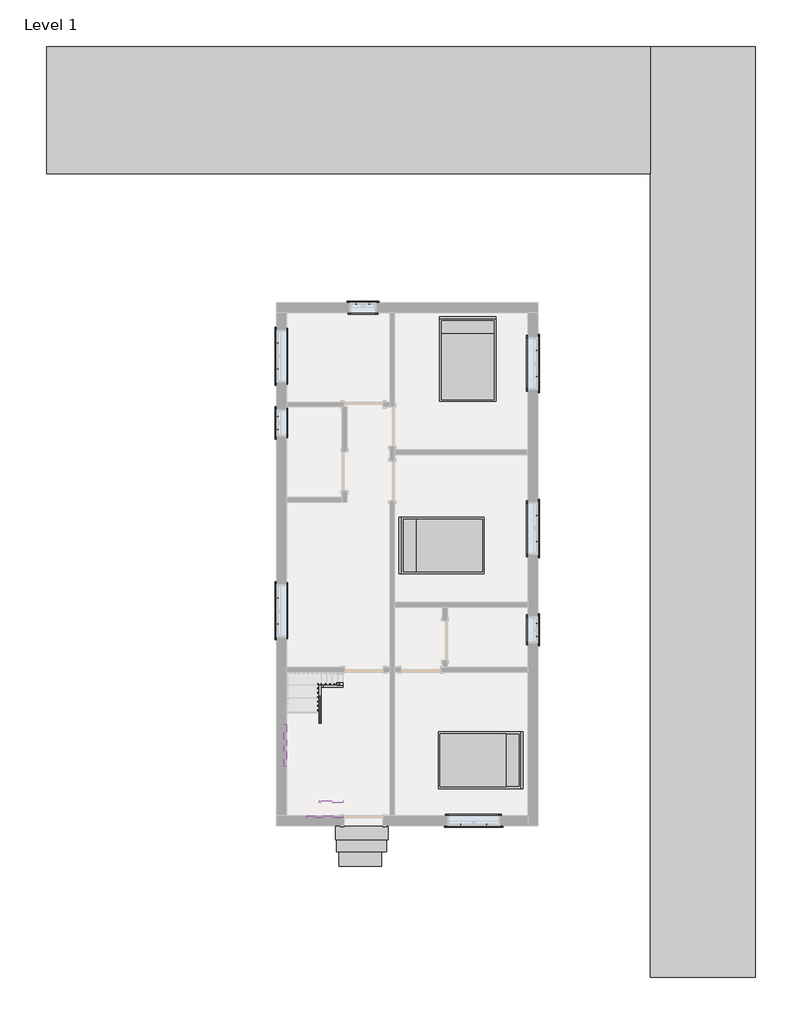
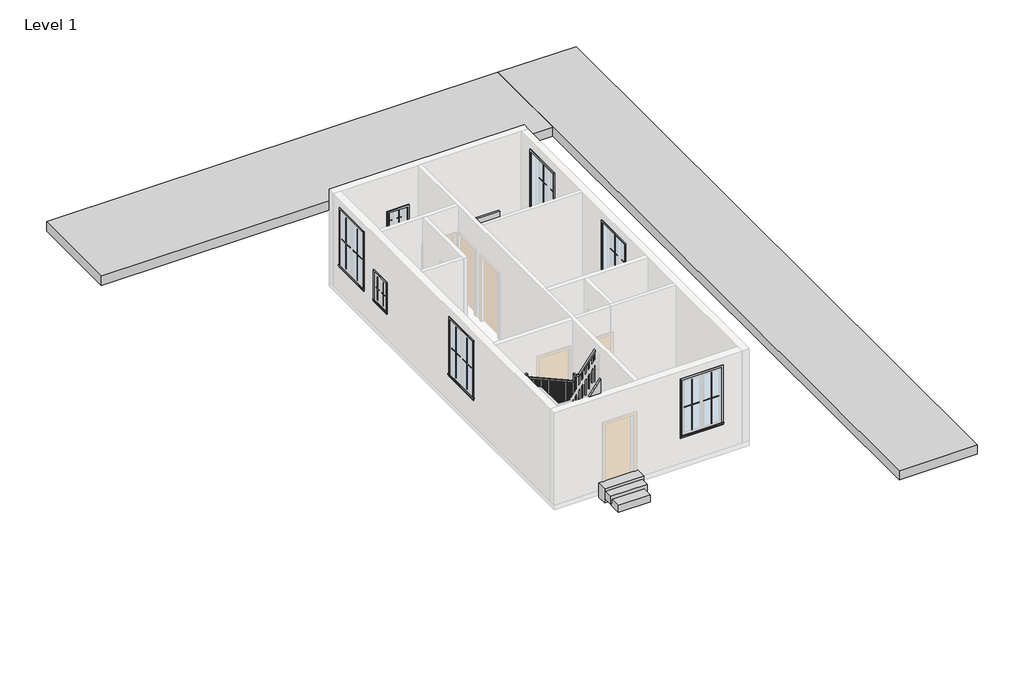
# One storey, part 2 of 2: 34 proxies, 6 members, 3 furniture elements, 1 railing.
"""IFC4 building model written with IfcOpenShell, lengths in millimetres."""

from ifc_helpers import new_model, si_unit, frame, origin, place, context, project, spatial, polyline, outline, extrude, faceted_brep, transform, mapped, element, save
from components import generic_models_1_generic_models_1_22b824c4, generic_models_2_generic_models_2_8981c4c3, muntin_pattern_2x2_muntin_pattern_2x2_2b4d9f72, muntin_pattern_2x2_muntin_pattern_2x2_ef995ed3, muntin_pattern_2x2_muntin_pattern_2x2_53152e2c, muntin_pattern_2x2_muntin_pattern_2x2_e8f3e573, trim_window_exterior_flat_with_sill_b7e4d11c, trim_window_exterior_flat_with_sill_a665a915, trim_window_interior_flat_picture_frame_936b8d2a, trim_window_interior_flat_picture_frame_d485c387, bed_17739_bed_17739_15c61121

model = new_model("IFC4")

# Units and contexts
model_context = context("Model", 3, world=origin())
ifc_project = project(units=[si_unit("LENGTHUNIT", "METRE", prefix="MILLI")], contexts=[model_context])

# Site, building, storey
site = spatial("IfcSite", under=ifc_project)
building = spatial("IfcBuilding", under=site)
storey = spatial("IfcBuildingStorey", under=building, Name="Level 1", Elevation=0.0)

# Proxies
placement = place(None, origin())
generic_models_1_generic_models_1_shape = generic_models_1_generic_models_1_22b824c4(model_context)
element("IfcBuildingElementProxy", 1, Name="Generic Models 1 : Generic Models 1", ObjectType="Generic Models 1 : Generic Models 1", at=placement, inside=storey, context=model_context, shape_type="MappedRepresentation", body=[
    mapped(generic_models_1_generic_models_1_shape, transform((0.0, 0.0, 0.0), x_axis=(1.0, 0.0, 0.0), y_axis=(0.0, 1.0, 0.0), z_axis=(0.0, 0.0, 1.0))),
])
generic_models_2_generic_models_2_shape = generic_models_2_generic_models_2_8981c4c3(model_context)
element("IfcBuildingElementProxy", 2, Name="Generic Models 2 : Generic Models 2", ObjectType="Generic Models 2 : Generic Models 2", at=placement, inside=storey, context=model_context, shape_type="MappedRepresentation", body=[
    mapped(generic_models_2_generic_models_2_shape, transform((0.0, 0.0, 0.0), x_axis=(1.0, 0.0, 0.0), y_axis=(0.0, 1.0, 0.0), z_axis=(0.0, 0.0, 1.0))),
])
muntin_pattern_2x2_muntin_pattern_2x2_shape = muntin_pattern_2x2_muntin_pattern_2x2_2b4d9f72(model_context)
element("IfcBuildingElementProxy", 3, Name="Muntin Pattern_2x2 : Muntin Pattern_2x2", ObjectType="Muntin Pattern_2x2 : Muntin Pattern_2x2", at=placement, inside=storey, context=model_context, shape_type="MappedRepresentation", body=[
    mapped(muntin_pattern_2x2_muntin_pattern_2x2_shape, transform((1533.525, 12679.3625, 984.25), x_axis=(0.0, 1.0, 0.0), y_axis=(-1.0, 0.0, 0.0), z_axis=(0.0, 0.0, 1.0))),
])
element("IfcBuildingElementProxy", 4, Name="Muntin Pattern_2x2 : Muntin Pattern_2x2", ObjectType="Muntin Pattern_2x2 : Muntin Pattern_2x2", at=placement, inside=storey, context=model_context, shape_type="MappedRepresentation", body=[
    mapped(muntin_pattern_2x2_muntin_pattern_2x2_shape, transform((7610.475, 13117.5125, 984.25), x_axis=(0.0, -1.0, 0.0), y_axis=(1.0, 0.0, 0.0), z_axis=(0.0, 0.0, 1.0))),
])
element("IfcBuildingElementProxy", 5, Name="Muntin Pattern_2x2 : Muntin Pattern_2x2", ObjectType="Muntin Pattern_2x2 : Muntin Pattern_2x2", at=placement, inside=storey, context=model_context, shape_type="MappedRepresentation", body=[
    mapped(muntin_pattern_2x2_muntin_pattern_2x2_shape, transform((7610.475, 9263.0625, 984.25), x_axis=(0.0, -1.0, 0.0), y_axis=(1.0, 0.0, 0.0), z_axis=(0.0, 0.0, 1.0))),
])
element("IfcBuildingElementProxy", 6, Name="Muntin Pattern_2x2 : Muntin Pattern_2x2", ObjectType="Muntin Pattern_2x2 : Muntin Pattern_2x2", at=placement, inside=storey, context=model_context, shape_type="MappedRepresentation", body=[
    mapped(muntin_pattern_2x2_muntin_pattern_2x2_shape, transform((6424.6125, 2041.525, 984.25), x_axis=(-1.0, 0.0, 0.0), y_axis=(0.0, -1.0, 0.0), z_axis=(0.0, 0.0, 1.0))),
])
element("IfcBuildingElementProxy", 7, Name="Muntin Pattern_2x2 : Muntin Pattern_2x2", ObjectType="Muntin Pattern_2x2 : Muntin Pattern_2x2", at=placement, inside=storey, context=model_context, shape_type="MappedRepresentation", body=[
    mapped(muntin_pattern_2x2_muntin_pattern_2x2_shape, transform((1533.525, 6738.9375, 984.25), x_axis=(0.0, 1.0, 0.0), y_axis=(-1.0, 0.0, 0.0), z_axis=(0.0, 0.0, 1.0))),
])
muntin_pattern_2x2_muntin_pattern_2x2_2_shape = muntin_pattern_2x2_muntin_pattern_2x2_ef995ed3(model_context)
element("IfcBuildingElementProxy", 8, Name="Muntin Pattern_2x2 : Muntin Pattern_2x2", ObjectType="Muntin Pattern_2x2 : Muntin Pattern_2x2", at=placement, inside=storey, context=model_context, shape_type="MappedRepresentation", body=[
    mapped(muntin_pattern_2x2_muntin_pattern_2x2_2_shape, transform((1533.525, 13285.7875, 984.25), x_axis=(0.0, -1.0, 0.0), y_axis=(1.0, 0.0, 0.0), z_axis=(0.0, 0.0, 1.0))),
])
element("IfcBuildingElementProxy", 9, Name="Muntin Pattern_2x2 : Muntin Pattern_2x2", ObjectType="Muntin Pattern_2x2 : Muntin Pattern_2x2", at=placement, inside=storey, context=model_context, shape_type="MappedRepresentation", body=[
    mapped(muntin_pattern_2x2_muntin_pattern_2x2_2_shape, transform((7610.475, 12511.0875, 984.25), x_axis=(0.0, 1.0, 0.0), y_axis=(-1.0, 0.0, 0.0), z_axis=(0.0, 0.0, 1.0))),
])
element("IfcBuildingElementProxy", 10, Name="Muntin Pattern_2x2 : Muntin Pattern_2x2", ObjectType="Muntin Pattern_2x2 : Muntin Pattern_2x2", at=placement, inside=storey, context=model_context, shape_type="MappedRepresentation", body=[
    mapped(muntin_pattern_2x2_muntin_pattern_2x2_2_shape, transform((7610.475, 8656.6375, 984.25), x_axis=(0.0, 1.0, 0.0), y_axis=(-1.0, 0.0, 0.0), z_axis=(0.0, 0.0, 1.0))),
])
element("IfcBuildingElementProxy", 11, Name="Muntin Pattern_2x2 : Muntin Pattern_2x2", ObjectType="Muntin Pattern_2x2 : Muntin Pattern_2x2", at=placement, inside=storey, context=model_context, shape_type="MappedRepresentation", body=[
    mapped(muntin_pattern_2x2_muntin_pattern_2x2_2_shape, transform((5818.1875, 2041.525, 984.25), x_axis=(1.0, 0.0, 0.0), y_axis=(0.0, 1.0, 0.0), z_axis=(0.0, 0.0, 1.0))),
])
element("IfcBuildingElementProxy", 12, Name="Muntin Pattern_2x2 : Muntin Pattern_2x2", ObjectType="Muntin Pattern_2x2 : Muntin Pattern_2x2", at=placement, inside=storey, context=model_context, shape_type="MappedRepresentation", body=[
    mapped(muntin_pattern_2x2_muntin_pattern_2x2_2_shape, transform((1533.525, 7345.3625, 984.25), x_axis=(0.0, -1.0, 0.0), y_axis=(1.0, 0.0, 0.0), z_axis=(0.0, 0.0, 1.0))),
])
muntin_pattern_2x2_muntin_pattern_2x2_3_shape = muntin_pattern_2x2_muntin_pattern_2x2_53152e2c(model_context)
element("IfcBuildingElementProxy", 13, Name="Muntin Pattern_2x2 : Muntin Pattern_2x2", ObjectType="Muntin Pattern_2x2 : Muntin Pattern_2x2", at=placement, inside=storey, context=model_context, shape_type="MappedRepresentation", body=[
    mapped(muntin_pattern_2x2_muntin_pattern_2x2_3_shape, transform((7610.475, 6748.4625, 984.25), x_axis=(0.0, -1.0, 0.0), y_axis=(1.0, 0.0, 0.0), z_axis=(0.0, 0.0, 1.0))),
])
element("IfcBuildingElementProxy", 14, Name="Muntin Pattern_2x2 : Muntin Pattern_2x2", ObjectType="Muntin Pattern_2x2 : Muntin Pattern_2x2", at=placement, inside=storey, context=model_context, shape_type="MappedRepresentation", body=[
    mapped(muntin_pattern_2x2_muntin_pattern_2x2_3_shape, transform((1533.525, 11272.8375, 984.25), x_axis=(0.0, 1.0, 0.0), y_axis=(-1.0, 0.0, 0.0), z_axis=(0.0, 0.0, 1.0))),
])
element("IfcBuildingElementProxy", 15, Name="Muntin Pattern_2x2 : Muntin Pattern_2x2", ObjectType="Muntin Pattern_2x2 : Muntin Pattern_2x2", at=placement, inside=storey, context=model_context, shape_type="MappedRepresentation", body=[
    mapped(muntin_pattern_2x2_muntin_pattern_2x2_3_shape, transform((3386.1375, 14214.475, 984.25), x_axis=(1.0, 0.0, 0.0), y_axis=(0.0, 1.0, 0.0), z_axis=(0.0, 0.0, 1.0))),
])
muntin_pattern_2x2_muntin_pattern_2x2_4_shape = muntin_pattern_2x2_muntin_pattern_2x2_e8f3e573(model_context)
element("IfcBuildingElementProxy", 16, Name="Muntin Pattern_2x2 : Muntin Pattern_2x2", ObjectType="Muntin Pattern_2x2 : Muntin Pattern_2x2", at=placement, inside=storey, context=model_context, shape_type="MappedRepresentation", body=[
    mapped(muntin_pattern_2x2_muntin_pattern_2x2_4_shape, transform((7610.475, 6446.8375, 984.25), x_axis=(0.0, 1.0, 0.0), y_axis=(-1.0, 0.0, 0.0), z_axis=(0.0, 0.0, 1.0))),
])
element("IfcBuildingElementProxy", 17, Name="Muntin Pattern_2x2 : Muntin Pattern_2x2", ObjectType="Muntin Pattern_2x2 : Muntin Pattern_2x2", at=placement, inside=storey, context=model_context, shape_type="MappedRepresentation", body=[
    mapped(muntin_pattern_2x2_muntin_pattern_2x2_4_shape, transform((1533.525, 11574.4625, 984.25), x_axis=(0.0, -1.0, 0.0), y_axis=(1.0, 0.0, 0.0), z_axis=(0.0, 0.0, 1.0))),
])
element("IfcBuildingElementProxy", 18, Name="Muntin Pattern_2x2 : Muntin Pattern_2x2", ObjectType="Muntin Pattern_2x2 : Muntin Pattern_2x2", at=placement, inside=storey, context=model_context, shape_type="MappedRepresentation", body=[
    mapped(muntin_pattern_2x2_muntin_pattern_2x2_4_shape, transform((3687.7625, 14214.475, 984.25), x_axis=(-1.0, 0.0, 0.0), y_axis=(0.0, -1.0, 0.0), z_axis=(0.0, 0.0, 1.0))),
])
trim_window_exterior_flat_with_sill_shape = trim_window_exterior_flat_with_sill_b7e4d11c(model_context)
element("IfcBuildingElementProxy", 19, Name="Trim-Window-Exterior-Flat : with Sill", ObjectType="Trim-Window-Exterior-Flat : with Sill", at=placement, inside=storey, context=model_context, shape_type="MappedRepresentation", body=[
    mapped(trim_window_exterior_flat_with_sill_shape, transform((1524.0, 12982.575, 2743.2), x_axis=(0.0, -1.0, 0.0), y_axis=(0.0, 0.0, 1.0), z_axis=(-1.0, 0.0, 0.0))),
])
element("IfcBuildingElementProxy", 20, Name="Trim-Window-Exterior-Flat : with Sill", ObjectType="Trim-Window-Exterior-Flat : with Sill", at=placement, inside=storey, context=model_context, shape_type="MappedRepresentation", body=[
    mapped(trim_window_exterior_flat_with_sill_shape, transform((7620.0, 12814.3, 2743.2), x_axis=(0.0, 1.0, 0.0), y_axis=(0.0, 0.0, 1.0), z_axis=(1.0, 0.0, 0.0))),
])
element("IfcBuildingElementProxy", 21, Name="Trim-Window-Exterior-Flat : with Sill", ObjectType="Trim-Window-Exterior-Flat : with Sill", at=placement, inside=storey, context=model_context, shape_type="MappedRepresentation", body=[
    mapped(trim_window_exterior_flat_with_sill_shape, transform((7620.0, 8959.85, 2743.2), x_axis=(0.0, 1.0, 0.0), y_axis=(0.0, 0.0, 1.0), z_axis=(1.0, 0.0, 0.0))),
])
element("IfcBuildingElementProxy", 22, Name="Trim-Window-Exterior-Flat : with Sill", ObjectType="Trim-Window-Exterior-Flat : with Sill", at=placement, inside=storey, context=model_context, shape_type="MappedRepresentation", body=[
    mapped(trim_window_exterior_flat_with_sill_shape, transform((6121.4, 2032.0, 2743.2), x_axis=(1.0, 0.0, 0.0), y_axis=(0.0, 0.0, 1.0), z_axis=(0.0, -1.0, 0.0))),
])
element("IfcBuildingElementProxy", 23, Name="Trim-Window-Exterior-Flat : with Sill", ObjectType="Trim-Window-Exterior-Flat : with Sill", at=placement, inside=storey, context=model_context, shape_type="MappedRepresentation", body=[
    mapped(trim_window_exterior_flat_with_sill_shape, transform((1524.0, 7042.15, 2743.2), x_axis=(0.0, -1.0, 0.0), y_axis=(0.0, 0.0, 1.0), z_axis=(-1.0, 0.0, 0.0))),
])
trim_window_exterior_flat_with_sill_2_shape = trim_window_exterior_flat_with_sill_a665a915(model_context)
element("IfcBuildingElementProxy", 24, Name="Trim-Window-Exterior-Flat : with Sill", ObjectType="Trim-Window-Exterior-Flat : with Sill", at=placement, inside=storey, context=model_context, shape_type="MappedRepresentation", body=[
    mapped(trim_window_exterior_flat_with_sill_2_shape, transform((7620.0, 6597.65, 1828.8), x_axis=(0.0, 1.0, 0.0), y_axis=(0.0, 0.0, 1.0), z_axis=(1.0, 0.0, 0.0))),
])
element("IfcBuildingElementProxy", 25, Name="Trim-Window-Exterior-Flat : with Sill", ObjectType="Trim-Window-Exterior-Flat : with Sill", at=placement, inside=storey, context=model_context, shape_type="MappedRepresentation", body=[
    mapped(trim_window_exterior_flat_with_sill_2_shape, transform((1524.0, 11423.65, 1828.8), x_axis=(0.0, -1.0, 0.0), y_axis=(0.0, 0.0, 1.0), z_axis=(-1.0, 0.0, 0.0))),
])
element("IfcBuildingElementProxy", 26, Name="Trim-Window-Exterior-Flat : with Sill", ObjectType="Trim-Window-Exterior-Flat : with Sill", at=placement, inside=storey, context=model_context, shape_type="MappedRepresentation", body=[
    mapped(trim_window_exterior_flat_with_sill_2_shape, transform((3536.95, 14224.0, 1828.8), x_axis=(-1.0, 0.0, 0.0), y_axis=(0.0, 0.0, 1.0), z_axis=(0.0, 1.0, 0.0))),
])
trim_window_interior_flat_picture_frame_shape = trim_window_interior_flat_picture_frame_936b8d2a(model_context)
element("IfcBuildingElementProxy", 27, Name="Trim-Window-Interior-Flat : Picture Frame", ObjectType="Trim-Window-Interior-Flat : Picture Frame", at=placement, inside=storey, context=model_context, shape_type="MappedRepresentation", body=[
    mapped(trim_window_interior_flat_picture_frame_shape, transform((1752.6, 12982.575, 2743.2), x_axis=(0.0, 1.0, 0.0), y_axis=(0.0, 0.0, 1.0), z_axis=(1.0, 0.0, 0.0))),
])
element("IfcBuildingElementProxy", 28, Name="Trim-Window-Interior-Flat : Picture Frame", ObjectType="Trim-Window-Interior-Flat : Picture Frame", at=placement, inside=storey, context=model_context, shape_type="MappedRepresentation", body=[
    mapped(trim_window_interior_flat_picture_frame_shape, transform((7391.4, 12814.3, 2743.2), x_axis=(0.0, -1.0, 0.0), y_axis=(0.0, 0.0, 1.0), z_axis=(-1.0, 0.0, 0.0))),
])
element("IfcBuildingElementProxy", 29, Name="Trim-Window-Interior-Flat : Picture Frame", ObjectType="Trim-Window-Interior-Flat : Picture Frame", at=placement, inside=storey, context=model_context, shape_type="MappedRepresentation", body=[
    mapped(trim_window_interior_flat_picture_frame_shape, transform((7391.4, 8959.85, 2743.2), x_axis=(0.0, -1.0, 0.0), y_axis=(0.0, 0.0, 1.0), z_axis=(-1.0, 0.0, 0.0))),
])
element("IfcBuildingElementProxy", 30, Name="Trim-Window-Interior-Flat : Picture Frame", ObjectType="Trim-Window-Interior-Flat : Picture Frame", at=placement, inside=storey, context=model_context, shape_type="MappedRepresentation", body=[
    mapped(trim_window_interior_flat_picture_frame_shape, transform((6121.4, 2260.6, 2743.2), x_axis=(-1.0, 0.0, 0.0), y_axis=(0.0, 0.0, 1.0), z_axis=(0.0, 1.0, 0.0))),
])
element("IfcBuildingElementProxy", 31, Name="Trim-Window-Interior-Flat : Picture Frame", ObjectType="Trim-Window-Interior-Flat : Picture Frame", at=placement, inside=storey, context=model_context, shape_type="MappedRepresentation", body=[
    mapped(trim_window_interior_flat_picture_frame_shape, transform((1752.6, 7042.15, 2743.2), x_axis=(0.0, 1.0, 0.0), y_axis=(0.0, 0.0, 1.0), z_axis=(1.0, 0.0, 0.0))),
])
trim_window_interior_flat_picture_frame_2_shape = trim_window_interior_flat_picture_frame_d485c387(model_context)
element("IfcBuildingElementProxy", 32, Name="Trim-Window-Interior-Flat : Picture Frame", ObjectType="Trim-Window-Interior-Flat : Picture Frame", at=placement, inside=storey, context=model_context, shape_type="MappedRepresentation", body=[
    mapped(trim_window_interior_flat_picture_frame_2_shape, transform((7391.4, 6597.65, 1828.8), x_axis=(0.0, -1.0, 0.0), y_axis=(0.0, 0.0, 1.0), z_axis=(-1.0, 0.0, 0.0))),
])
element("IfcBuildingElementProxy", 33, Name="Trim-Window-Interior-Flat : Picture Frame", ObjectType="Trim-Window-Interior-Flat : Picture Frame", at=placement, inside=storey, context=model_context, shape_type="MappedRepresentation", body=[
    mapped(trim_window_interior_flat_picture_frame_2_shape, transform((1752.6, 11423.65, 1828.8), x_axis=(0.0, 1.0, 0.0), y_axis=(0.0, 0.0, 1.0), z_axis=(1.0, 0.0, 0.0))),
])
element("IfcBuildingElementProxy", 34, Name="Trim-Window-Interior-Flat : Picture Frame", ObjectType="Trim-Window-Interior-Flat : Picture Frame", at=placement, inside=storey, context=model_context, shape_type="MappedRepresentation", body=[
    mapped(trim_window_interior_flat_picture_frame_2_shape, transform((3536.95, 13995.4, 1828.8), x_axis=(1.0, 0.0, 0.0), y_axis=(0.0, 0.0, 1.0), z_axis=(0.0, -1.0, 0.0))),
])

# Furniture
bed_17739_bed_17739_shape = bed_17739_bed_17739_15c61121(model_context)
element("IfcFurniture", 35, ObjectType="Bed_17739 : Bed_17739", at=placement, inside=storey, context=model_context, shape_type="MappedRepresentation", body=[
    mapped(bed_17739_bed_17739_shape, transform((6261.1, 3556.0, 0.0), x_axis=(0.0, -1.0, 0.0), y_axis=(1.0, 0.0, 0.0), z_axis=(0.0, 0.0, 1.0))),
])
element("IfcFurniture", 36, ObjectType="Bed_17739 : Bed_17739", at=placement, inside=storey, context=model_context, shape_type="MappedRepresentation", body=[
    mapped(bed_17739_bed_17739_shape, transform((5397.5, 8566.15, 0.0), x_axis=(0.0, 1.0, 0.0), y_axis=(-1.0, 0.0, 0.0), z_axis=(0.0, 0.0, 1.0))),
])
element("IfcFurniture", 37, ObjectType="Bed_17739 : Bed_17739", at=placement, inside=storey, context=model_context, shape_type="MappedRepresentation", body=[
    mapped(bed_17739_bed_17739_shape, transform((5981.7, 12890.5, 0.0), x_axis=(1.0, 0.0, 0.0), y_axis=(0.0, 1.0, 0.0), z_axis=(0.0, 0.0, 1.0))),
])

# Members
element("IfcMember", 38, ObjectType="Stringer - 2\" Width", at=placement, inside=storey, context=model_context, shape_type="SweptSolid", body=[
    extrude(outline(polyline([(0.0, 3073.4), (318.3960727, 3073.4), (1054.2650614, 2604.2835197), (1054.2650614, 2565.4), (548.2495371, 2565.4), (0.0, 2914.9090799), (0.0, 3073.4)])), frame((0.0, 5257.8, 0.0), z_axis=(0.0, 1.0, 0.0), x_axis=(0.0, 0.0, 1.0)), (0.0, 0.0, 1.0), 50.8),
])
element("IfcMember", 39, ObjectType="Stringer - 2\" Width", at=placement, inside=storey, context=model_context, shape_type="SweptSolid", body=[
    extrude(outline(polyline([(5308.6, 1054.2650614), (5308.6, 705.5863873), (2616.2, 2201.3641651), (2616.2, 2550.0428392), (5308.6, 1054.2650614)])), frame((2514.6, 0.0, 0.0), z_axis=(1.0, 0.0, 0.0), x_axis=(0.0, 1.0, 0.0)), (0.0, 0.0, 1.0), 50.8),
])
element("IfcMember", 40, ObjectType="Stringer - 2\" Width", at=placement, inside=storey, context=model_context, shape_type="SweptSolid", body=[
    extrude(outline(polyline([(2718.9450923, 2514.6), (2229.5863873, 2514.6), (2229.5863873, 2564.102242), (3028.4848312, 3073.4), (3595.4941119, 3073.4), (2718.9450923, 2514.6)])), frame((0.0, 2565.4, 0.0), z_axis=(0.0, 1.0, 0.0), x_axis=(0.0, 0.0, 1.0)), (0.0, 0.0, 1.0), 50.8),
])
element("IfcMember", 41, ObjectType="Stringer - 2\" Width", at=placement, inside=storey, context=model_context, shape_type="SweptSolid", body=[
    extrude(outline(polyline([(0.0, 3073.4), (309.0333333, 3073.4), (884.9317281, 2641.4762039), (884.9317281, 2260.4762039), (0.0, 2924.175), (0.0, 3073.4)])), frame((0.0, 5613.4, 0.0), z_axis=(0.0, 1.0, 0.0), x_axis=(0.0, 0.0, 1.0)), (0.0, 0.0, 1.0), 50.8),
])
element("IfcMember", 42, ObjectType="Stringer - 2\" Width", at=placement, inside=storey, context=model_context, shape_type="SweptSolid", body=[
    extrude(outline(polyline([(3766.8754972, 1562.1), (3401.1154972, 1765.3), (4028.7371106, 1765.3), (4394.4971106, 1562.1), (3766.8754972, 1562.1)])), frame((1701.8, 0.0, 0.0), z_axis=(1.0, 0.0, 0.0), x_axis=(0.0, 1.0, 0.0)), (0.0, 0.0, 1.0), 50.8),
])
element("IfcMember", 43, ObjectType="Stringer - 2\" Width", at=placement, inside=storey, context=model_context, shape_type="SweptSolid", body=[
    extrude(outline(polyline([(2398.9197207, 2608.8147905), (3018.3666667, 3073.4), (3526.3666667, 3073.4), (2398.9197207, 2227.8147905), (2398.9197207, 2608.8147905)])), frame((0.0, 2209.8, 0.0), z_axis=(0.0, 1.0, 0.0), x_axis=(0.0, 0.0, 1.0)), (0.0, 0.0, 1.0), 50.8),
])

# Railing
element("IfcRailing", 44, ObjectType="Handrail - Rectangular", at=placement, inside=storey, context=model_context, shape_type="SolidModel", body=[
    faceted_brep([(3073.4, 5308.6, 1083.7333333), (3073.4, 5308.6, 999.0666667), (3073.4, 5359.4, 999.0666667), (3073.4, 5359.4, 1083.7333333), (2590.8, 5308.6, 1727.2), (2540.0, 5308.6, 1710.2666667), (2540.0, 5359.4, 1710.2666667), (2590.8, 5359.4, 1727.2), (2590.8, 5308.6, 1972.7333333), (2540.0, 5308.6, 1921.9333333), (2540.0, 5359.4, 1921.9333333), (2590.8, 5359.4, 1972.7333333), (2514.6, 5308.6, 1972.7333333), (2514.6, 5308.6, 1921.9333333), (2463.8, 5359.4, 1921.9333333), (2463.8, 5359.4, 1972.7333333), (2514.6, 5232.4, 1972.7333333), (2514.6, 5219.2363978, 1921.9333333), (2463.8, 5219.2363978, 1921.9333333), (2463.8, 5232.4, 1972.7333333), (2514.6, 2641.6, 3412.0666667), (2514.6, 2590.8, 3382.1757765), (2463.8, 2590.8, 3382.1757765), (2463.8, 2641.6, 3412.0666667), (2514.6, 2641.6, 3657.6), (2514.6, 2590.8, 3606.8), (2463.8, 2590.8, 3606.8), (2463.8, 2641.6, 3657.6), (2514.6, 2565.4, 3657.6), (2514.6, 2565.4, 3606.8), (2463.8, 2514.6, 3606.8), (2463.8, 2514.6, 3657.6), (2590.8, 2565.4, 3657.6), (2616.2, 2565.4, 3606.8), (2616.2, 2514.6, 3606.8), (2590.8, 2514.6, 3657.6), (3073.4, 2565.4, 4301.0666667), (3073.4, 2514.6, 4301.0666667), (3073.4, 2514.6, 4216.4), (3073.4, 2565.4, 4216.4)], [[[0, 1, 2, 3]], [[1, 0, 4, 5]], [[2, 1, 5, 6]], [[3, 2, 6, 7]], [[0, 3, 7, 4]], [[5, 4, 8, 9]], [[6, 5, 9, 10]], [[7, 6, 10, 11]], [[4, 7, 11, 8]], [[9, 8, 12, 13]], [[10, 9, 13, 14]], [[11, 10, 14, 15]], [[8, 11, 15, 12]], [[13, 12, 16, 17]], [[14, 13, 17, 18]], [[15, 14, 18, 19]], [[12, 15, 19, 16]], [[17, 16, 20, 21]], [[18, 17, 21, 22]], [[19, 18, 22, 23]], [[16, 19, 23, 20]], [[21, 20, 24, 25]], [[22, 21, 25, 26]], [[23, 22, 26, 27]], [[20, 23, 27, 24]], [[25, 24, 28, 29]], [[26, 25, 29, 30]], [[27, 26, 30, 31]], [[24, 27, 31, 28]], [[29, 28, 32, 33]], [[30, 29, 33, 34]], [[31, 30, 34, 35]], [[28, 31, 35, 32]], [[36, 37, 38, 39]], [[33, 32, 36, 39]], [[34, 33, 39, 38]], [[35, 34, 38, 37]], [[32, 35, 37, 36]]]),
    extrude(outline(polyline([(4102.1, 2987.675), (3217.3333333, 2987.675), (3217.3333333, 3006.725), (4127.5, 3006.725), (4102.1, 2987.675)])), frame((0.0, 2530.475, 0.0), z_axis=(0.0, 1.0, 0.0), x_axis=(0.0, 0.0, 1.0)), (0.0, 0.0, 1.0), 19.05),
    extrude(outline(polyline([(3966.6333333, 2886.075), (3048.0, 2886.075), (3048.0, 2905.125), (3992.0333333, 2905.125), (3966.6333333, 2886.075)])), frame((0.0, 2530.475, 0.0), z_axis=(0.0, 1.0, 0.0), x_axis=(0.0, 0.0, 1.0)), (0.0, 0.0, 1.0), 19.05),
    extrude(outline(polyline([(3831.1666667, 2784.475), (2878.6666667, 2784.475), (2878.6666667, 2803.525), (3856.5666667, 2803.525), (3831.1666667, 2784.475)])), frame((0.0, 2530.475, 0.0), z_axis=(0.0, 1.0, 0.0), x_axis=(0.0, 0.0, 1.0)), (0.0, 0.0, 1.0), 19.05),
    extrude(outline(polyline([(3695.7, 2682.875), (2878.6666667, 2682.875), (2878.6666667, 2701.925), (3721.1, 2701.925), (3695.7, 2682.875)])), frame((0.0, 2530.475, 0.0), z_axis=(0.0, 1.0, 0.0), x_axis=(0.0, 0.0, 1.0)), (0.0, 0.0, 1.0), 19.05),
    extrude(outline(polyline([(3560.2333333, 2581.275), (2709.3333333, 2581.275), (2709.3333333, 2600.325), (3585.6333333, 2600.325), (3560.2333333, 2581.275)])), frame((0.0, 2530.475, 0.0), z_axis=(0.0, 1.0, 0.0), x_axis=(0.0, 0.0, 1.0)), (0.0, 0.0, 1.0), 19.05),
    extrude(outline(polyline([(2498.725, 2600.325), (2498.725, 2581.275), (2479.675, 2581.275), (2479.675, 2600.325), (2498.725, 2600.325)])), frame((0.0, 0.0, 2370.6666667), z_axis=(0.0, 0.0, 1.0), x_axis=(1.0, 0.0, 0.0)), (0.0, 0.0, 1.0), 1236.1333333),
    extrude(outline(polyline([(2701.925, 3320.4396654), (2701.925, 2370.6666667), (2682.875, 2370.6666667), (2682.875, 3331.0229988), (2701.925, 3320.4396654)])), frame((2479.675, 0.0, 0.0), z_axis=(1.0, 0.0, 0.0), x_axis=(0.0, 1.0, 0.0)), (0.0, 0.0, 1.0), 19.05),
    extrude(outline(polyline([(2803.525, 3263.995221), (2803.525, 2370.6666667), (2784.475, 2370.6666667), (2784.475, 3274.5785543), (2803.525, 3263.995221)])), frame((2479.675, 0.0, 0.0), z_axis=(1.0, 0.0, 0.0), x_axis=(0.0, 1.0, 0.0)), (0.0, 0.0, 1.0), 19.05),
    extrude(outline(polyline([(2905.125, 3207.5507765), (2905.125, 2201.3333333), (2886.075, 2201.3333333), (2886.075, 3218.1341099), (2905.125, 3207.5507765)])), frame((2479.675, 0.0, 0.0), z_axis=(1.0, 0.0, 0.0), x_axis=(0.0, 1.0, 0.0)), (0.0, 0.0, 1.0), 19.05),
    extrude(outline(polyline([(3006.725, 3151.1063321), (3006.725, 2201.3333333), (2987.675, 2201.3333333), (2987.675, 3161.6896654), (3006.725, 3151.1063321)])), frame((2479.675, 0.0, 0.0), z_axis=(1.0, 0.0, 0.0), x_axis=(0.0, 1.0, 0.0)), (0.0, 0.0, 1.0), 19.05),
    extrude(outline(polyline([(3108.325, 3094.6618876), (3108.325, 2201.3333333), (3089.275, 2201.3333333), (3089.275, 3105.245221), (3108.325, 3094.6618876)])), frame((2479.675, 0.0, 0.0), z_axis=(1.0, 0.0, 0.0), x_axis=(0.0, 1.0, 0.0)), (0.0, 0.0, 1.0), 19.05),
    extrude(outline(polyline([(3209.925, 3038.2174432), (3209.925, 2032.0), (3190.875, 2032.0), (3190.875, 3048.8007765), (3209.925, 3038.2174432)])), frame((2479.675, 0.0, 0.0), z_axis=(1.0, 0.0, 0.0), x_axis=(0.0, 1.0, 0.0)), (0.0, 0.0, 1.0), 19.05),
    extrude(outline(polyline([(3311.525, 2981.7729988), (3311.525, 2032.0), (3292.475, 2032.0), (3292.475, 2992.3563321), (3311.525, 2981.7729988)])), frame((2479.675, 0.0, 0.0), z_axis=(1.0, 0.0, 0.0), x_axis=(0.0, 1.0, 0.0)), (0.0, 0.0, 1.0), 19.05),
    extrude(outline(polyline([(3413.125, 2925.3285543), (3413.125, 2032.0), (3394.075, 2032.0), (3394.075, 2935.9118876), (3413.125, 2925.3285543)])), frame((2479.675, 0.0, 0.0), z_axis=(1.0, 0.0, 0.0), x_axis=(0.0, 1.0, 0.0)), (0.0, 0.0, 1.0), 19.05),
    extrude(outline(polyline([(3514.725, 2868.8841099), (3514.725, 1862.6666667), (3495.675, 1862.6666667), (3495.675, 2879.4674432), (3514.725, 2868.8841099)])), frame((2479.675, 0.0, 0.0), z_axis=(1.0, 0.0, 0.0), x_axis=(0.0, 1.0, 0.0)), (0.0, 0.0, 1.0), 19.05),
    extrude(outline(polyline([(3616.325, 2812.4396654), (3616.325, 1862.6666667), (3597.275, 1862.6666667), (3597.275, 2823.0229988), (3616.325, 2812.4396654)])), frame((2479.675, 0.0, 0.0), z_axis=(1.0, 0.0, 0.0), x_axis=(0.0, 1.0, 0.0)), (0.0, 0.0, 1.0), 19.05),
    extrude(outline(polyline([(3717.925, 2755.995221), (3717.925, 1862.6666667), (3698.875, 1862.6666667), (3698.875, 2766.5785543), (3717.925, 2755.995221)])), frame((2479.675, 0.0, 0.0), z_axis=(1.0, 0.0, 0.0), x_axis=(0.0, 1.0, 0.0)), (0.0, 0.0, 1.0), 19.05),
    extrude(outline(polyline([(3819.525, 2699.5507765), (3819.525, 1693.3333333), (3800.475, 1693.3333333), (3800.475, 2710.1341099), (3819.525, 2699.5507765)])), frame((2479.675, 0.0, 0.0), z_axis=(1.0, 0.0, 0.0), x_axis=(0.0, 1.0, 0.0)), (0.0, 0.0, 1.0), 19.05),
    extrude(outline(polyline([(3921.125, 2643.1063321), (3921.125, 1693.3333333), (3902.075, 1693.3333333), (3902.075, 2653.6896654), (3921.125, 2643.1063321)])), frame((2479.675, 0.0, 0.0), z_axis=(1.0, 0.0, 0.0), x_axis=(0.0, 1.0, 0.0)), (0.0, 0.0, 1.0), 19.05),
    extrude(outline(polyline([(4022.725, 2586.6618876), (4022.725, 1693.3333333), (4003.675, 1693.3333333), (4003.675, 2597.245221), (4022.725, 2586.6618876)])), frame((2479.675, 0.0, 0.0), z_axis=(1.0, 0.0, 0.0), x_axis=(0.0, 1.0, 0.0)), (0.0, 0.0, 1.0), 19.05),
    extrude(outline(polyline([(4124.325, 2530.2174432), (4124.325, 1524.0), (4105.275, 1524.0), (4105.275, 2540.8007765), (4124.325, 2530.2174432)])), frame((2479.675, 0.0, 0.0), z_axis=(1.0, 0.0, 0.0), x_axis=(0.0, 1.0, 0.0)), (0.0, 0.0, 1.0), 19.05),
    extrude(outline(polyline([(4225.925, 2473.7729988), (4225.925, 1524.0), (4206.875, 1524.0), (4206.875, 2484.3563321), (4225.925, 2473.7729988)])), frame((2479.675, 0.0, 0.0), z_axis=(1.0, 0.0, 0.0), x_axis=(0.0, 1.0, 0.0)), (0.0, 0.0, 1.0), 19.05),
    extrude(outline(polyline([(4327.525, 2417.3285543), (4327.525, 1524.0), (4308.475, 1524.0), (4308.475, 2427.9118876), (4327.525, 2417.3285543)])), frame((2479.675, 0.0, 0.0), z_axis=(1.0, 0.0, 0.0), x_axis=(0.0, 1.0, 0.0)), (0.0, 0.0, 1.0), 19.05),
    extrude(outline(polyline([(4429.125, 2360.8841099), (4429.125, 1354.6666667), (4410.075, 1354.6666667), (4410.075, 2371.4674432), (4429.125, 2360.8841099)])), frame((2479.675, 0.0, 0.0), z_axis=(1.0, 0.0, 0.0), x_axis=(0.0, 1.0, 0.0)), (0.0, 0.0, 1.0), 19.05),
    extrude(outline(polyline([(4530.725, 2304.4396654), (4530.725, 1354.6666667), (4511.675, 1354.6666667), (4511.675, 2315.0229988), (4530.725, 2304.4396654)])), frame((2479.675, 0.0, 0.0), z_axis=(1.0, 0.0, 0.0), x_axis=(0.0, 1.0, 0.0)), (0.0, 0.0, 1.0), 19.05),
    extrude(outline(polyline([(4632.325, 2247.995221), (4632.325, 1354.6666667), (4613.275, 1354.6666667), (4613.275, 2258.5785543), (4632.325, 2247.995221)])), frame((2479.675, 0.0, 0.0), z_axis=(1.0, 0.0, 0.0), x_axis=(0.0, 1.0, 0.0)), (0.0, 0.0, 1.0), 19.05),
    extrude(outline(polyline([(4733.925, 2191.5507765), (4733.925, 1185.3333333), (4714.875, 1185.3333333), (4714.875, 2202.1341099), (4733.925, 2191.5507765)])), frame((2479.675, 0.0, 0.0), z_axis=(1.0, 0.0, 0.0), x_axis=(0.0, 1.0, 0.0)), (0.0, 0.0, 1.0), 19.05),
    extrude(outline(polyline([(4835.525, 2135.1063321), (4835.525, 1185.3333333), (4816.475, 1185.3333333), (4816.475, 2145.6896654), (4835.525, 2135.1063321)])), frame((2479.675, 0.0, 0.0), z_axis=(1.0, 0.0, 0.0), x_axis=(0.0, 1.0, 0.0)), (0.0, 0.0, 1.0), 19.05),
    extrude(outline(polyline([(4937.125, 2078.6618876), (4937.125, 1185.3333333), (4918.075, 1185.3333333), (4918.075, 2089.245221), (4937.125, 2078.6618876)])), frame((2479.675, 0.0, 0.0), z_axis=(1.0, 0.0, 0.0), x_axis=(0.0, 1.0, 0.0)), (0.0, 0.0, 1.0), 19.05),
    extrude(outline(polyline([(5038.725, 2022.2174432), (5038.725, 1016.0), (5019.675, 1016.0), (5019.675, 2032.8007765), (5038.725, 2022.2174432)])), frame((2479.675, 0.0, 0.0), z_axis=(1.0, 0.0, 0.0), x_axis=(0.0, 1.0, 0.0)), (0.0, 0.0, 1.0), 19.05),
    extrude(outline(polyline([(5140.325, 1965.7729988), (5140.325, 1016.0), (5121.275, 1016.0), (5121.275, 1976.3563321), (5140.325, 1965.7729988)])), frame((2479.675, 0.0, 0.0), z_axis=(1.0, 0.0, 0.0), x_axis=(0.0, 1.0, 0.0)), (0.0, 0.0, 1.0), 19.05),
    extrude(outline(polyline([(5241.925, 1909.3285543), (5241.925, 1016.0), (5222.875, 1016.0), (5222.875, 1919.9118876), (5241.925, 1909.3285543)])), frame((2479.675, 0.0, 0.0), z_axis=(1.0, 0.0, 0.0), x_axis=(0.0, 1.0, 0.0)), (0.0, 0.0, 1.0), 19.05),
    extrude(outline(polyline([(2574.925, 5324.475), (2555.875, 5324.475), (2555.875, 5343.525), (2574.925, 5343.525), (2574.925, 5324.475)])), frame((0.0, 0.0, 846.6666667), z_axis=(0.0, 0.0, 1.0), x_axis=(1.0, 0.0, 0.0)), (0.0, 0.0, 1.0), 1075.2666667),
    extrude(outline(polyline([(1553.6333333, 2657.475), (677.3333333, 2657.475), (677.3333333, 2676.525), (1528.2333333, 2676.525), (1553.6333333, 2657.475)])), frame((0.0, 5324.475, 0.0), z_axis=(0.0, 1.0, 0.0), x_axis=(0.0, 0.0, 1.0)), (0.0, 0.0, 1.0), 19.05),
    extrude(outline(polyline([(1418.1666667, 2759.075), (508.0, 2759.075), (508.0, 2778.125), (1392.7666667, 2778.125), (1418.1666667, 2759.075)])), frame((0.0, 5324.475, 0.0), z_axis=(0.0, 1.0, 0.0), x_axis=(0.0, 0.0, 1.0)), (0.0, 0.0, 1.0), 19.05),
    extrude(outline(polyline([(1282.7, 2860.675), (338.6666667, 2860.675), (338.6666667, 2879.725), (1257.3, 2879.725), (1282.7, 2860.675)])), frame((0.0, 5324.475, 0.0), z_axis=(0.0, 1.0, 0.0), x_axis=(0.0, 0.0, 1.0)), (0.0, 0.0, 1.0), 19.05),
    extrude(outline(polyline([(1147.2333333, 2962.275), (169.3333333, 2962.275), (169.3333333, 2981.325), (1121.8333333, 2981.325), (1147.2333333, 2962.275)])), frame((0.0, 5324.475, 0.0), z_axis=(0.0, 1.0, 0.0), x_axis=(0.0, 0.0, 1.0)), (0.0, 0.0, 1.0), 19.05),
    extrude(outline(polyline([(2498.725, 2549.525), (2498.725, 2530.475), (2479.675, 2530.475), (2479.675, 2549.525), (2498.725, 2549.525)])), frame((0.0, 0.0, 2540.0), z_axis=(0.0, 0.0, 1.0), x_axis=(1.0, 0.0, 0.0)), (0.0, 0.0, 1.0), 1066.8),
    extrude(outline(polyline([(2498.725, 5324.475), (2479.675, 5324.475), (2479.675, 5343.525), (2498.725, 5343.525), (2498.725, 5324.475)])), frame((0.0, 0.0, 846.6666667), z_axis=(0.0, 0.0, 1.0), x_axis=(1.0, 0.0, 0.0)), (0.0, 0.0, 1.0), 1075.2666667),
    extrude(outline(polyline([(4191.0, 3054.35), (3217.3333333, 3054.35), (3217.3333333, 3073.4), (4216.4, 3073.4), (4191.0, 3054.35)])), frame((0.0, 2530.475, 0.0), z_axis=(0.0, 1.0, 0.0), x_axis=(0.0, 0.0, 1.0)), (0.0, 0.0, 1.0), 19.05),
    extrude(outline(polyline([(1024.4666667, 3054.35), (169.3333333, 3054.35), (169.3333333, 3073.4), (999.0666667, 3073.4), (1024.4666667, 3054.35)])), frame((0.0, 5324.475, 0.0), z_axis=(0.0, 1.0, 0.0), x_axis=(0.0, 0.0, 1.0)), (0.0, 0.0, 1.0), 19.05),
])

save(model, "model.ifc")

# Revit data of these elements
# Type "Muntin Pattern_2x2 : Muntin Pattern_2x2"
#   Width [instance default] = 4' - 0"
#   Thickness = 0' - 0 1/2"
#   Height [instance default] = 4' - 0"
#   Distance = 0' - 0 3/4"
#   Interior Material [instance default] = none
#   Exterior Material [instance default] = none
#   Default Elevation = 0
# Type "Trim-Window-Exterior-Flat : with Sill"
#   Trim Width = 0' - 2 1/4"
#   Trim Thickness_Picture Frame = 0' - 1 1/4"
#   Trim Thickness_with Sill = 0' - 0 3/4"
#   Sill Thickness = 0' - 1 1/4"
#   Opening Width [instance default] = 2' - 0"
#   Opening Height [instance default] = 3' - 0"
#   Default Elevation = 4' - 0"
#   Sill = yes
#   Picture Frame = no
#   Trim Material [instance default] = none
# Type "Trim-Window-Interior-Flat : Picture Frame"
#   Trim Thickness_Picture Frame = 0' - 1 1/4"
#   Trim Width = 0' - 2 1/4"
#   Trim Thickness_with Sill = 0' - 0 3/4"
#   Sill Thickness = 0' - 1 1/4"
#   Opening Width [instance default] = 2' - 0"
#   Opening Height [instance default] = 3' - 0"
#   Default Elevation = 4' - 0"
#   Sill = no
#   Picture Frame = yes
#   Trim Material [instance default] = none
# Type "Bed_17739 : Bed_17739"
#   Default Elevation = 0
# Type "Handrail - Rectangular"
#   Assembly Code = "C2010400"
#   built-in parameter 1008612 = 0.0416667 (stored number, unit not read)
#   built-in parameter 1008611 = 0.0416667 (stored number, unit not read)
#   built-in parameter 1008609 = 0.333333 (stored number, unit not read)
#   built-in parameter 1008604 = 0.166667 (stored number, unit not read)
#   built-in parameter 1008603 = 0.166667 (stored number, unit not read)
#   Railing Height = 3' - 0"
#   built-in parameter 1008630 = 2
#   built-in parameter 1008610 = 2
#   built-in parameter 1008618 = Baluster - Square : 3/4"
# Element 1 (IfcBuildingElementProxy, "Generic Models 1 : Generic Models 1")
#   Phase Created = New Construction
#   Materials on its faces: "Door - Panel"
# Element 2 (IfcBuildingElementProxy, "Generic Models 2 : Generic Models 2")
#   Phase Created = New Construction
# Elements 3, 4, 5, 6, 7, 8, 9, 10, 11, 12 (IfcBuildingElementProxy, "Muntin Pattern_2x2 : Muntin Pattern_2x2")
#   Width = 1' - 6 5/8"
#   Height = 5' - 6 1/2"
#   Interior Material = Wood - Stained
#   Exterior Material = Clad - White
#   Phase Created = New Construction
#   Materials on its faces: "Clad - White", "Wood - Stained"
# Elements 13, 14, 15, 16, 17, 18 (IfcBuildingElementProxy, "Muntin Pattern_2x2 : Muntin Pattern_2x2")
#   Width = 0' - 6 5/8"
#   Height = 2' - 6 1/2"
#   Interior Material = Wood - Stained
#   Exterior Material = Clad - White
#   Phase Created = New Construction
#   Materials on its faces: "Clad - White", "Wood - Stained"
# Elements 19, 20, 21, 22, 23 (IfcBuildingElementProxy, "Trim-Window-Exterior-Flat : with Sill")
#   Opening Width = 4' - 0"
#   Opening Height = 6' - 0"
#   Trim Material = Clad - White
#   Phase Created = New Construction
#   Materials on its faces: "Clad - White"
# Elements 24, 25, 26 (IfcBuildingElementProxy, "Trim-Window-Exterior-Flat : with Sill")
#   Opening Width = 2' - 0"
#   Opening Height = 3' - 0"
#   Trim Material = Clad - White
#   Phase Created = New Construction
#   Materials on its faces: "Clad - White"
# Elements 27, 28, 29, 30, 31 (IfcBuildingElementProxy, "Trim-Window-Interior-Flat : Picture Frame")
#   Opening Width = 4' - 0"
#   Opening Height = 6' - 0"
#   Trim Material = Wood - Stained
#   Phase Created = New Construction
#   Materials on its faces: "Wood - Stained"
# Elements 32, 33, 34 (IfcBuildingElementProxy, "Trim-Window-Interior-Flat : Picture Frame")
#   Opening Width = 2' - 0"
#   Opening Height = 3' - 0"
#   Trim Material = Wood - Stained
#   Phase Created = New Construction
#   Materials on its faces: "Wood - Stained"
# Elements 35, 36, 37 (IfcFurniture, "Bed_17739 : Bed_17739")
#   Phase Created = New Construction
#   Materials on its faces: "legs", "sheets", "bed frame", "Blanket"
# Elements 38, 39, 40, 41, 42, 43 (IfcMember, "Stringer - 2\" Width")
#   Phase Created = New Construction
# Element 44 (IfcRailing, "Handrail - Rectangular")
#   Phase Created = New Construction
# Materials
#   "Door - Panel": class "Wood", colour RGB 210 159 95, transparency 0, Cost = 0
#   "Clad - White": class "Wood", colour RGB 242 242 238, transparency 0, Cost = 0
#   "Wood - Stained": class "Wood", colour RGB 224 178 126, transparency 0, Cost = 0
#   "legs": colour RGB 90 73 37, transparency 0, Cost = 0
#   "sheets": colour RGB 200 195 176, transparency 0, Cost = 0
#   "bed frame": colour RGB 90 73 37, transparency 0, Cost = 0
#   "Blanket": class "System", colour RGB 59 0 1, transparency 0, Cost = 0
